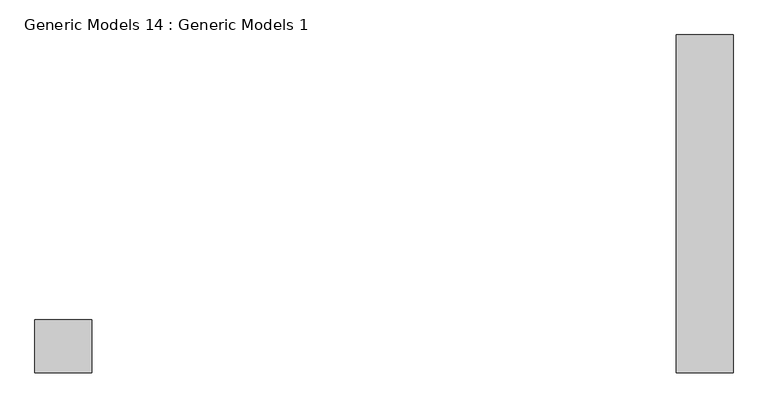
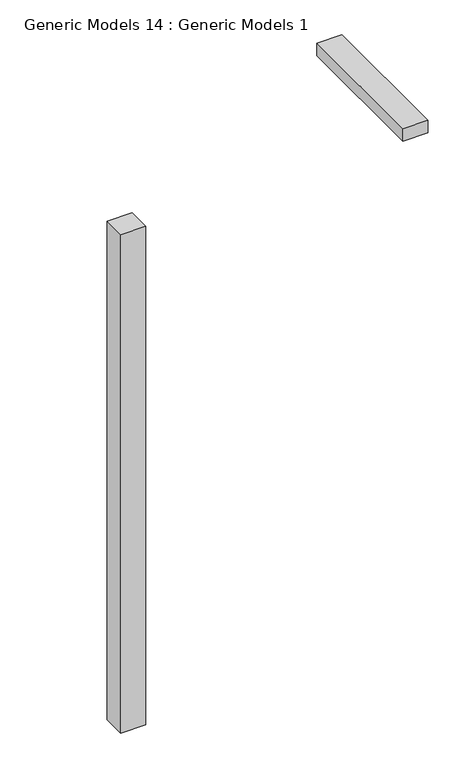
"""IFC4 building model written with IfcOpenShell, lengths in millimetres: proxy geometry, Generic Models 14 : Generic Models 1."""

from ifc_helpers import new_model, si_unit, frame, origin, origin_with_axes, place, context, project, spatial, polyline, outline, extrude, source, transform, mapped, element, save


def generic_models_14_generic_models_1_67c994ca(model_context):
    return source(origin(), model_context, "Body", "SweptSolid", [
        extrude(outline(polyline([(-9698.5642415, -4709.7273102), (-9546.1642415, -4709.7273102), (-9546.1642415, -5613.7098142), (-9698.5642415, -5613.7098142), (-9698.5642415, -4709.7273102)])), frame((0.0, 0.0, 3200.4), z_axis=(0.0, 0.0, 1.0), x_axis=(1.0, 0.0, 0.0)), (0.0, 0.0, 1.0), 79.9931522),
        extrude(outline(polyline([(-11413.9852694, -5471.7273102), (-11261.5852694, -5471.7273102), (-11261.5852694, -5613.7098142), (-11413.9852694, -5613.7098142), (-11413.9852694, -5471.7273102)])), origin_with_axes(), (0.0, 0.0, 1.0), 3200.4),
    ])


if __name__ == "__main__":
    model = new_model("IFC4")
    model_context = context("Model", 3, world=origin())
    ifc_project = project(units=[si_unit("LENGTHUNIT", "METRE", prefix="MILLI")], contexts=[model_context])
    site = spatial("IfcSite", under=ifc_project)
    building = spatial("IfcBuilding", under=site)
    placement = place(None, origin())
    generic_models_14_generic_models_1_shape = generic_models_14_generic_models_1_67c994ca(model_context)
    element("IfcBuildingElementProxy", 1, Name="Generic Models 14 : Generic Models 1", ObjectType="Generic Models 14 : Generic Models 1", at=placement, inside=building, context=model_context, shape_type="MappedRepresentation", body=[
        mapped(generic_models_14_generic_models_1_shape, transform((0.0, 0.0, 0.0), x_axis=(1.0, 0.0, 0.0), y_axis=(0.0, 1.0, 0.0), z_axis=(0.0, 0.0, 1.0))),
    ])
    save(model, "model.ifc")
